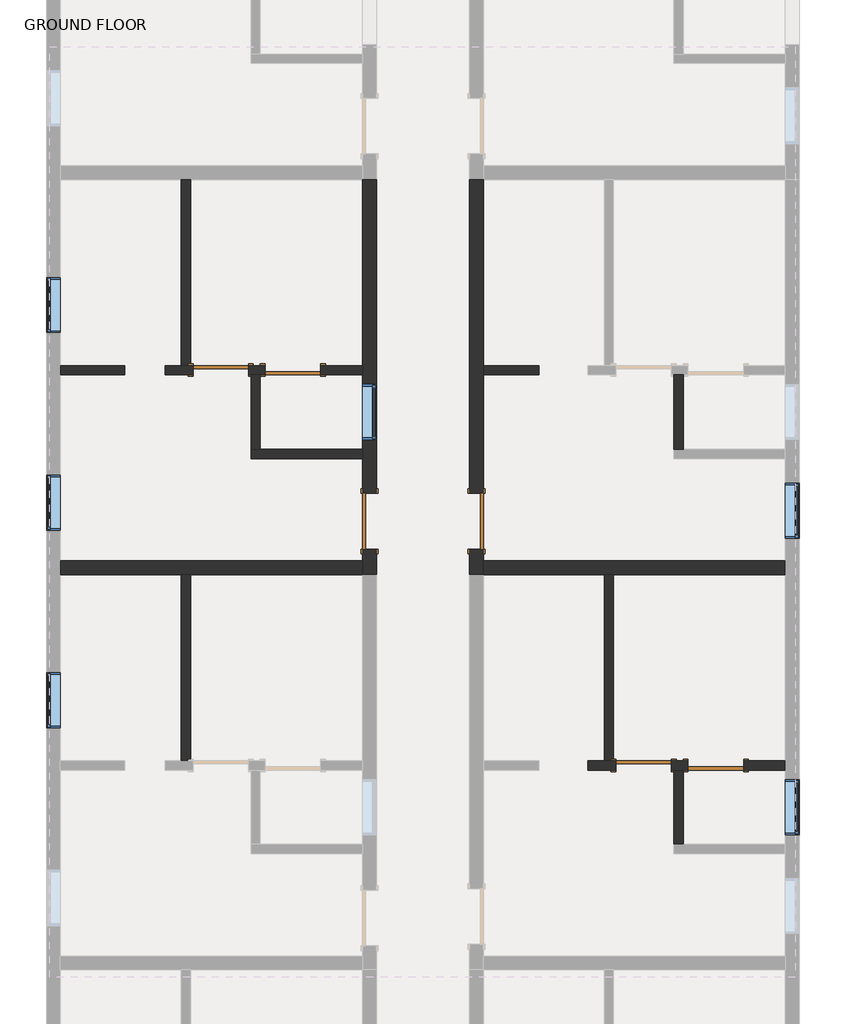
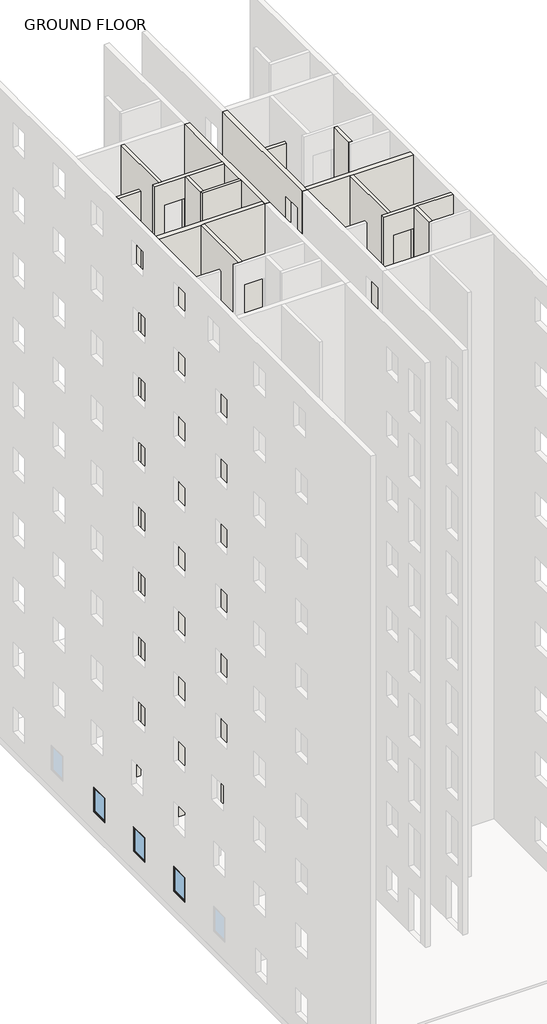
# One storey, part 5 of 7: 15 walls, 6 doors, 6 windows.
"""IFC4 building model written with IfcOpenShell, lengths in millimetres."""

from ifc_helpers import new_model, si_unit, origin, origin_with_axes, place, context, project, spatial, polyline, outline, extrude, faceted_brep, transform, mapped, element, save
from components import door_686f89d2, door_16372e1c, door_a90ba1ad, door_0ca8825f, window_c1f32544

model = new_model("IFC4")

# Units and contexts
model_context = context("Model", 3, world=origin())
ifc_project = project(units=[si_unit("LENGTHUNIT", "METRE", prefix="MILLI")], contexts=[model_context])

# Site, building, storey
site = spatial("IfcSite", under=ifc_project)
building = spatial("IfcBuilding", under=site)
storey = spatial("IfcBuildingStorey", under=building, Name="GROUND FLOOR", Elevation=0.0)

# Doors
placement = place(None, origin())
door_shape = door_686f89d2(model_context)
element("IfcDoor", 1, ObjectType="Single-Flush : 36\" x 84\"", at=placement, inside=storey, context=model_context, shape_type="MappedRepresentation", body=[
    mapped(door_shape, transform((-9863.5902461, 5475.2710592, 0.0), x_axis=(-1.0, 0.0, 0.0), y_axis=(0.0, -1.0, 0.0), z_axis=(0.0, 0.0, 1.0))),
])
element("IfcDoor", 2, ObjectType="Single-Flush : 36\" x 84\"", at=placement, inside=storey, context=model_context, shape_type="MappedRepresentation", body=[
    mapped(door_shape, transform((-2929.3902461, -1001.7289408, 0.0), x_axis=(-1.0, 0.0, 0.0), y_axis=(0.0, -1.0, 0.0), z_axis=(0.0, 0.0, 1.0))),
])
door_2_shape = door_16372e1c(model_context)
element("IfcDoor", 3, ObjectType="Single-Flush : 36\" x 84\"", at=placement, inside=storey, context=model_context, shape_type="MappedRepresentation", body=[
    mapped(door_2_shape, transform((-8682.4902461, 5475.2710592, 0.0), x_axis=(-1.0, 0.0, 0.0), y_axis=(0.0, -1.0, 0.0), z_axis=(0.0, 0.0, 1.0))),
])
element("IfcDoor", 4, ObjectType="Single-Flush : 36\" x 84\"", at=placement, inside=storey, context=model_context, shape_type="MappedRepresentation", body=[
    mapped(door_2_shape, transform((-1748.2902461, -1001.7289408, 0.0), x_axis=(-1.0, 0.0, 0.0), y_axis=(0.0, -1.0, 0.0), z_axis=(0.0, 0.0, 1.0))),
])
door_3_shape = door_a90ba1ad(model_context)
element("IfcDoor", 5, ObjectType="Single-Flush : 36\" x 84\"", at=placement, inside=storey, context=model_context, shape_type="MappedRepresentation", body=[
    mapped(door_3_shape, transform((-7425.1902461, 2998.7710592, 0.0), x_axis=(0.0, -1.0, 0.0), y_axis=(1.0, 0.0, 0.0), z_axis=(0.0, 0.0, 1.0))),
])
door_4_shape = door_0ca8825f(model_context)
element("IfcDoor", 6, ObjectType="Single-Flush : 36\" x 84\"", at=placement, inside=storey, context=model_context, shape_type="MappedRepresentation", body=[
    mapped(door_4_shape, transform((-5672.5902461, 2998.7710592, 0.0), x_axis=(0.0, -1.0, 0.0), y_axis=(1.0, 0.0, 0.0), z_axis=(0.0, 0.0, 1.0))),
])

# Walls
element("IfcWall", 7, ObjectType="Generic - 8\"", at=placement, inside=storey, context=model_context, shape_type="Brep", body=[
    faceted_brep([(-5558.2902461, 2122.4710592, 0.0), (-5558.2902461, 2351.0710592, 0.0), (-5558.2902461, 2541.5710592, 0.0), (-5558.2902461, 2541.5710592, 2133.6), (-5558.2902461, 3455.9710592, 2133.6), (-5558.2902461, 3455.9710592, 0.0), (-5558.2902461, 5399.0710592, 0.0), (-5558.2902461, 5551.4710592, 0.0), (-5558.2902461, 8599.4710592, 0.0), (-5558.2902461, 8599.4710592, 32004.0), (-5558.2902461, 5551.4710592, 32004.0), (-5558.2902461, 5399.0710592, 32004.0), (-5558.2902461, 2351.0710592, 32004.0), (-5558.2902461, 2122.4710592, 32004.0), (-5558.2902461, 3455.9710592, 3200.4), (-5558.2902461, 2541.5710592, 3200.4), (-5558.2902461, 2541.5710592, 5334.0), (-5558.2902461, 3455.9710592, 5334.0), (-5558.2902461, 3455.9710592, 6400.8), (-5558.2902461, 2541.5710592, 6400.8), (-5558.2902461, 2541.5710592, 8534.4), (-5558.2902461, 3455.9710592, 8534.4), (-5558.2902461, 3455.9710592, 9601.2), (-5558.2902461, 2541.5710592, 9601.2), (-5558.2902461, 2541.5710592, 11734.8), (-5558.2902461, 3455.9710592, 11734.8), (-5558.2902461, 3455.9710592, 12801.6), (-5558.2902461, 2541.5710592, 12801.6), (-5558.2902461, 2541.5710592, 14935.2), (-5558.2902461, 3455.9710592, 14935.2), (-5558.2902461, 3455.9710592, 19202.4), (-5558.2902461, 2541.5710592, 19202.4), (-5558.2902461, 2541.5710592, 21336.0), (-5558.2902461, 3455.9710592, 21336.0), (-5558.2902461, 3455.9710592, 22402.8), (-5558.2902461, 2541.5710592, 22402.8), (-5558.2902461, 2541.5710592, 24536.4), (-5558.2902461, 3455.9710592, 24536.4), (-5558.2902461, 3455.9710592, 25603.2), (-5558.2902461, 2541.5710592, 25603.2), (-5558.2902461, 2541.5710592, 27736.8), (-5558.2902461, 3455.9710592, 27736.8), (-5558.2902461, 3455.9710592, 28803.6), (-5558.2902461, 2541.5710592, 28803.6), (-5558.2902461, 2541.5710592, 30937.2), (-5558.2902461, 3455.9710592, 30937.2), (-5786.8902461, 2541.5710592, 2133.6), (-5786.8902461, 2541.5710592, 0.0), (-5786.8902461, 2122.4710592, 0.0), (-5786.8902461, 2122.4710592, 32004.0), (-5786.8902461, 8599.4710592, 32004.0), (-5786.8902461, 8599.4710592, 0.0), (-5786.8902461, 3455.9710592, 0.0), (-5786.8902461, 3455.9710592, 2133.6), (-5786.8902461, 3455.9710592, 3200.4), (-5786.8902461, 3455.9710592, 5334.0), (-5786.8902461, 2541.5710592, 5334.0), (-5786.8902461, 2541.5710592, 3200.4), (-5786.8902461, 3455.9710592, 6400.8), (-5786.8902461, 3455.9710592, 8534.4), (-5786.8902461, 2541.5710592, 8534.4), (-5786.8902461, 2541.5710592, 6400.8), (-5786.8902461, 3455.9710592, 9601.2), (-5786.8902461, 3455.9710592, 11734.8), (-5786.8902461, 2541.5710592, 11734.8), (-5786.8902461, 2541.5710592, 9601.2), (-5786.8902461, 3455.9710592, 12801.6), (-5786.8902461, 3455.9710592, 14935.2), (-5786.8902461, 2541.5710592, 14935.2), (-5786.8902461, 2541.5710592, 12801.6), (-5786.8902461, 3455.9710592, 19202.4), (-5786.8902461, 3455.9710592, 21336.0), (-5786.8902461, 2541.5710592, 21336.0), (-5786.8902461, 2541.5710592, 19202.4), (-5786.8902461, 3455.9710592, 22402.8), (-5786.8902461, 3455.9710592, 24536.4), (-5786.8902461, 2541.5710592, 24536.4), (-5786.8902461, 2541.5710592, 22402.8), (-5786.8902461, 3455.9710592, 25603.2), (-5786.8902461, 3455.9710592, 27736.8), (-5786.8902461, 2541.5710592, 27736.8), (-5786.8902461, 2541.5710592, 25603.2), (-5786.8902461, 3455.9710592, 28803.6), (-5786.8902461, 3455.9710592, 30937.2), (-5786.8902461, 2541.5710592, 30937.2), (-5786.8902461, 2541.5710592, 28803.6)], [[[0, 1, 2, 3, 4, 5, 6, 7, 8, 9, 10, 11, 12, 13], [14, 15, 16, 17], [18, 19, 20, 21], [22, 23, 24, 25], [26, 27, 28, 29], [30, 31, 32, 33], [34, 35, 36, 37], [38, 39, 40, 41], [42, 43, 44, 45]], [[46, 47, 48, 49, 50, 51, 52, 53], [54, 55, 56, 57], [58, 59, 60, 61], [62, 63, 64, 65], [66, 67, 68, 69], [70, 71, 72, 73], [74, 75, 76, 77], [78, 79, 80, 81], [82, 83, 84, 85]], [[52, 51, 8, 7, 6, 5]], [[48, 47, 2, 1, 0]], [[13, 12, 11, 10, 9, 50, 49]], [[0, 13, 49, 48]], [[9, 8, 51, 50]], [[3, 2, 47, 46]], [[4, 3, 46, 53]], [[5, 4, 53, 52]], [[15, 14, 54, 57]], [[16, 15, 57, 56]], [[17, 16, 56, 55]], [[14, 17, 55, 54]], [[19, 18, 58, 61]], [[20, 19, 61, 60]], [[21, 20, 60, 59]], [[18, 21, 59, 58]], [[23, 22, 62, 65]], [[24, 23, 65, 64]], [[25, 24, 64, 63]], [[22, 25, 63, 62]], [[27, 26, 66, 69]], [[28, 27, 69, 68]], [[29, 28, 68, 67]], [[26, 29, 67, 66]], [[31, 30, 70, 73]], [[32, 31, 73, 72]], [[33, 32, 72, 71]], [[30, 33, 71, 70]], [[35, 34, 74, 77]], [[36, 35, 77, 76]], [[37, 36, 76, 75]], [[34, 37, 75, 74]], [[39, 38, 78, 81]], [[40, 39, 81, 80]], [[41, 40, 80, 79]], [[38, 41, 79, 78]], [[43, 42, 82, 85]], [[44, 43, 85, 84]], [[45, 44, 84, 83]], [[42, 45, 83, 82]]]),
])
element("IfcWall", 8, ObjectType="INNER WALL 2", at=placement, inside=storey, context=model_context, shape_type="SweptSolid", body=[
    extrude(outline(polyline([(-2281.6902461, 5399.0710592), (-2281.6902461, 4179.8710592), (-2434.0902461, 4179.8710592), (-2434.0902461, 5399.0710592), (-2281.6902461, 5399.0710592)])), origin_with_axes(), (0.0, 0.0, 1.0), 32004.0),
])
element("IfcWall", 9, ObjectType="INNER WALL 2", at=placement, inside=storey, context=model_context, shape_type="Brep", body=[
    faceted_brep([(-2472.1902461, -1077.9289408, 0.0), (-2434.0902461, -1077.9289408, 0.0), (-2281.6902461, -1077.9289408, 0.0), (-2205.4902461, -1077.9289408, 0.0), (-2205.4902461, -1077.9289408, 2133.6), (-1291.0902461, -1077.9289408, 2133.6), (-1291.0902461, -1077.9289408, 0.0), (-605.2902461, -1077.9289408, 0.0), (-605.2902461, -1077.9289408, 32004.0), (-2281.6902461, -1077.9289408, 32004.0), (-2434.0902461, -1077.9289408, 32004.0), (-3843.7902461, -1077.9289408, 32004.0), (-3843.7902461, -1077.9289408, 0.0), (-3386.5902461, -1077.9289408, 0.0), (-3386.5902461, -1077.9289408, 2133.6), (-2472.1902461, -1077.9289408, 2133.6), (-1291.0902461, -1077.9289408, 3200.4), (-2205.4902461, -1077.9289408, 3200.4), (-2205.4902461, -1077.9289408, 5334.0), (-1291.0902461, -1077.9289408, 5334.0), (-2472.1902461, -1077.9289408, 3200.4), (-3386.5902461, -1077.9289408, 3200.4), (-3386.5902461, -1077.9289408, 5334.0), (-2472.1902461, -1077.9289408, 5334.0), (-2472.1902461, -1077.9289408, 6400.8), (-3386.5902461, -1077.9289408, 6400.8), (-3386.5902461, -1077.9289408, 8534.4), (-2472.1902461, -1077.9289408, 8534.4), (-1291.0902461, -1077.9289408, 6400.8), (-2205.4902461, -1077.9289408, 6400.8), (-2205.4902461, -1077.9289408, 8534.4), (-1291.0902461, -1077.9289408, 8534.4), (-2472.1902461, -1077.9289408, 9601.2), (-3386.5902461, -1077.9289408, 9601.2), (-3386.5902461, -1077.9289408, 11734.8), (-2472.1902461, -1077.9289408, 11734.8), (-1291.0902461, -1077.9289408, 9601.2), (-2205.4902461, -1077.9289408, 9601.2), (-2205.4902461, -1077.9289408, 11734.8), (-1291.0902461, -1077.9289408, 11734.8), (-1291.0902461, -1077.9289408, 12801.6), (-2205.4902461, -1077.9289408, 12801.6), (-2205.4902461, -1077.9289408, 14935.2), (-1291.0902461, -1077.9289408, 14935.2), (-2472.1902461, -1077.9289408, 12801.6), (-3386.5902461, -1077.9289408, 12801.6), (-3386.5902461, -1077.9289408, 14935.2), (-2472.1902461, -1077.9289408, 14935.2), (-2472.1902461, -1077.9289408, 16002.0), (-3386.5902461, -1077.9289408, 16002.0), (-3386.5902461, -1077.9289408, 18135.6), (-2472.1902461, -1077.9289408, 18135.6), (-1291.0902461, -1077.9289408, 16002.0), (-2205.4902461, -1077.9289408, 16002.0), (-2205.4902461, -1077.9289408, 18135.6), (-1291.0902461, -1077.9289408, 18135.6), (-1291.0902461, -1077.9289408, 19202.4), (-2205.4902461, -1077.9289408, 19202.4), (-2205.4902461, -1077.9289408, 21336.0), (-1291.0902461, -1077.9289408, 21336.0), (-2472.1902461, -1077.9289408, 19202.4), (-3386.5902461, -1077.9289408, 19202.4), (-3386.5902461, -1077.9289408, 21336.0), (-2472.1902461, -1077.9289408, 21336.0), (-1291.0902461, -1077.9289408, 22402.8), (-2205.4902461, -1077.9289408, 22402.8), (-2205.4902461, -1077.9289408, 24536.4), (-1291.0902461, -1077.9289408, 24536.4), (-2472.1902461, -1077.9289408, 22402.8), (-3386.5902461, -1077.9289408, 22402.8), (-3386.5902461, -1077.9289408, 24536.4), (-2472.1902461, -1077.9289408, 24536.4), (-2472.1902461, -1077.9289408, 25603.2), (-3386.5902461, -1077.9289408, 25603.2), (-3386.5902461, -1077.9289408, 27736.8), (-2472.1902461, -1077.9289408, 27736.8), (-1291.0902461, -1077.9289408, 25603.2), (-2205.4902461, -1077.9289408, 25603.2), (-2205.4902461, -1077.9289408, 27736.8), (-1291.0902461, -1077.9289408, 27736.8), (-2472.1902461, -1077.9289408, 28803.6), (-3386.5902461, -1077.9289408, 28803.6), (-3386.5902461, -1077.9289408, 30937.2), (-2472.1902461, -1077.9289408, 30937.2), (-1291.0902461, -1077.9289408, 28803.6), (-2205.4902461, -1077.9289408, 28803.6), (-2205.4902461, -1077.9289408, 30937.2), (-1291.0902461, -1077.9289408, 30937.2), (-2205.4902461, -925.5289408, 2133.6), (-2205.4902461, -925.5289408, 0.0), (-2472.1902461, -925.5289408, 0.0), (-2472.1902461, -925.5289408, 2133.6), (-3386.5902461, -925.5289408, 2133.6), (-3386.5902461, -925.5289408, 0.0), (-3424.6902461, -925.5289408, 0.0), (-3577.0902461, -925.5289408, 0.0), (-3843.7902461, -925.5289408, 0.0), (-3843.7902461, -925.5289408, 32004.0), (-3577.0902461, -925.5289408, 32004.0), (-3424.6902461, -925.5289408, 32004.0), (-605.2902461, -925.5289408, 32004.0), (-605.2902461, -925.5289408, 0.0), (-1291.0902461, -925.5289408, 0.0), (-1291.0902461, -925.5289408, 2133.6), (-1291.0902461, -925.5289408, 3200.4), (-1291.0902461, -925.5289408, 5334.0), (-2205.4902461, -925.5289408, 5334.0), (-2205.4902461, -925.5289408, 3200.4), (-2472.1902461, -925.5289408, 3200.4), (-2472.1902461, -925.5289408, 5334.0), (-3386.5902461, -925.5289408, 5334.0), (-3386.5902461, -925.5289408, 3200.4), (-2472.1902461, -925.5289408, 6400.8), (-2472.1902461, -925.5289408, 8534.4), (-3386.5902461, -925.5289408, 8534.4), (-3386.5902461, -925.5289408, 6400.8), (-1291.0902461, -925.5289408, 6400.8), (-1291.0902461, -925.5289408, 8534.4), (-2205.4902461, -925.5289408, 8534.4), (-2205.4902461, -925.5289408, 6400.8), (-2472.1902461, -925.5289408, 9601.2), (-2472.1902461, -925.5289408, 11734.8), (-3386.5902461, -925.5289408, 11734.8), (-3386.5902461, -925.5289408, 9601.2), (-1291.0902461, -925.5289408, 9601.2), (-1291.0902461, -925.5289408, 11734.8), (-2205.4902461, -925.5289408, 11734.8), (-2205.4902461, -925.5289408, 9601.2), (-1291.0902461, -925.5289408, 12801.6), (-1291.0902461, -925.5289408, 14935.2), (-2205.4902461, -925.5289408, 14935.2), (-2205.4902461, -925.5289408, 12801.6), (-2472.1902461, -925.5289408, 12801.6), (-2472.1902461, -925.5289408, 14935.2), (-3386.5902461, -925.5289408, 14935.2), (-3386.5902461, -925.5289408, 12801.6), (-2472.1902461, -925.5289408, 16002.0), (-2472.1902461, -925.5289408, 18135.6), (-3386.5902461, -925.5289408, 18135.6), (-3386.5902461, -925.5289408, 16002.0), (-1291.0902461, -925.5289408, 16002.0), (-1291.0902461, -925.5289408, 18135.6), (-2205.4902461, -925.5289408, 18135.6), (-2205.4902461, -925.5289408, 16002.0), (-1291.0902461, -925.5289408, 19202.4), (-1291.0902461, -925.5289408, 21336.0), (-2205.4902461, -925.5289408, 21336.0), (-2205.4902461, -925.5289408, 19202.4), (-2472.1902461, -925.5289408, 19202.4), (-2472.1902461, -925.5289408, 21336.0), (-3386.5902461, -925.5289408, 21336.0), (-3386.5902461, -925.5289408, 19202.4), (-1291.0902461, -925.5289408, 22402.8), (-1291.0902461, -925.5289408, 24536.4), (-2205.4902461, -925.5289408, 24536.4), (-2205.4902461, -925.5289408, 22402.8), (-2472.1902461, -925.5289408, 22402.8), (-2472.1902461, -925.5289408, 24536.4), (-3386.5902461, -925.5289408, 24536.4), (-3386.5902461, -925.5289408, 22402.8), (-2472.1902461, -925.5289408, 25603.2), (-2472.1902461, -925.5289408, 27736.8), (-3386.5902461, -925.5289408, 27736.8), (-3386.5902461, -925.5289408, 25603.2), (-1291.0902461, -925.5289408, 25603.2), (-1291.0902461, -925.5289408, 27736.8), (-2205.4902461, -925.5289408, 27736.8), (-2205.4902461, -925.5289408, 25603.2), (-2472.1902461, -925.5289408, 28803.6), (-2472.1902461, -925.5289408, 30937.2), (-3386.5902461, -925.5289408, 30937.2), (-3386.5902461, -925.5289408, 28803.6), (-1291.0902461, -925.5289408, 28803.6), (-1291.0902461, -925.5289408, 30937.2), (-2205.4902461, -925.5289408, 30937.2), (-2205.4902461, -925.5289408, 28803.6)], [[[0, 1, 2, 3, 4, 5, 6, 7, 8, 9, 10, 11, 12, 13, 14, 15], [16, 17, 18, 19], [20, 21, 22, 23], [24, 25, 26, 27], [28, 29, 30, 31], [32, 33, 34, 35], [36, 37, 38, 39], [40, 41, 42, 43], [44, 45, 46, 47], [48, 49, 50, 51], [52, 53, 54, 55], [56, 57, 58, 59], [60, 61, 62, 63], [64, 65, 66, 67], [68, 69, 70, 71], [72, 73, 74, 75], [76, 77, 78, 79], [80, 81, 82, 83], [84, 85, 86, 87]], [[88, 89, 90, 91, 92, 93, 94, 95, 96, 97, 98, 99, 100, 101, 102, 103], [104, 105, 106, 107], [108, 109, 110, 111], [112, 113, 114, 115], [116, 117, 118, 119], [120, 121, 122, 123], [124, 125, 126, 127], [128, 129, 130, 131], [132, 133, 134, 135], [136, 137, 138, 139], [140, 141, 142, 143], [144, 145, 146, 147], [148, 149, 150, 151], [152, 153, 154, 155], [156, 157, 158, 159], [160, 161, 162, 163], [164, 165, 166, 167], [168, 169, 170, 171], [172, 173, 174, 175]], [[96, 95, 94, 93, 13, 12]], [[102, 101, 7, 6]], [[90, 89, 3, 2, 1, 0]], [[11, 10, 9, 8, 100, 99, 98, 97]], [[12, 11, 97, 96]], [[8, 7, 101, 100]], [[14, 13, 93, 92]], [[15, 14, 92, 91]], [[0, 15, 91, 90]], [[4, 3, 89, 88]], [[5, 4, 88, 103]], [[6, 5, 103, 102]], [[17, 16, 104, 107]], [[18, 17, 107, 106]], [[19, 18, 106, 105]], [[16, 19, 105, 104]], [[21, 20, 108, 111]], [[22, 21, 111, 110]], [[23, 22, 110, 109]], [[20, 23, 109, 108]], [[25, 24, 112, 115]], [[26, 25, 115, 114]], [[27, 26, 114, 113]], [[24, 27, 113, 112]], [[29, 28, 116, 119]], [[30, 29, 119, 118]], [[31, 30, 118, 117]], [[28, 31, 117, 116]], [[33, 32, 120, 123]], [[34, 33, 123, 122]], [[35, 34, 122, 121]], [[32, 35, 121, 120]], [[37, 36, 124, 127]], [[38, 37, 127, 126]], [[39, 38, 126, 125]], [[36, 39, 125, 124]], [[41, 40, 128, 131]], [[42, 41, 131, 130]], [[43, 42, 130, 129]], [[40, 43, 129, 128]], [[45, 44, 132, 135]], [[46, 45, 135, 134]], [[47, 46, 134, 133]], [[44, 47, 133, 132]], [[49, 48, 136, 139]], [[50, 49, 139, 138]], [[51, 50, 138, 137]], [[48, 51, 137, 136]], [[53, 52, 140, 143]], [[54, 53, 143, 142]], [[55, 54, 142, 141]], [[52, 55, 141, 140]], [[57, 56, 144, 147]], [[58, 57, 147, 146]], [[59, 58, 146, 145]], [[56, 59, 145, 144]], [[61, 60, 148, 151]], [[62, 61, 151, 150]], [[63, 62, 150, 149]], [[60, 63, 149, 148]], [[65, 64, 152, 155]], [[66, 65, 155, 154]], [[67, 66, 154, 153]], [[64, 67, 153, 152]], [[69, 68, 156, 159]], [[70, 69, 159, 158]], [[71, 70, 158, 157]], [[68, 71, 157, 156]], [[73, 72, 160, 163]], [[74, 73, 163, 162]], [[75, 74, 162, 161]], [[72, 75, 161, 160]], [[77, 76, 164, 167]], [[78, 77, 167, 166]], [[79, 78, 166, 165]], [[76, 79, 165, 164]], [[81, 80, 168, 171]], [[82, 81, 171, 170]], [[83, 82, 170, 169]], [[80, 83, 169, 168]], [[85, 84, 172, 175]], [[86, 85, 175, 174]], [[87, 86, 174, 173]], [[84, 87, 173, 172]]]),
])
element("IfcWall", 10, ObjectType="INNER WALL 2", at=placement, inside=storey, context=model_context, shape_type="SweptSolid", body=[
    extrude(outline(polyline([(-3424.6902461, 2122.4710592), (-3424.6902461, -925.5289408), (-3577.0902461, -925.5289408), (-3577.0902461, 2122.4710592), (-3424.6902461, 2122.4710592)])), origin_with_axes(), (0.0, 0.0, 1.0), 32004.0),
])
element("IfcWall", 11, ObjectType="INNER WALL 2", at=placement, inside=storey, context=model_context, shape_type="SweptSolid", body=[
    extrude(outline(polyline([(-2281.6902461, -1077.9289408), (-2281.6902461, -2297.1289408), (-2434.0902461, -2297.1289408), (-2434.0902461, -1077.9289408), (-2281.6902461, -1077.9289408)])), origin_with_axes(), (0.0, 0.0, 1.0), 32004.0),
])
element("IfcWall", 12, ObjectType="INNER WALL 2", at=placement, inside=storey, context=model_context, shape_type="Brep", body=[
    faceted_brep([(-9406.3902461, 5399.0710592, 0.0), (-9368.2902461, 5399.0710592, 0.0), (-9215.8902461, 5399.0710592, 0.0), (-9139.6902461, 5399.0710592, 0.0), (-9139.6902461, 5399.0710592, 2133.6), (-8225.2902461, 5399.0710592, 2133.6), (-8225.2902461, 5399.0710592, 0.0), (-7539.4902461, 5399.0710592, 0.0), (-7539.4902461, 5399.0710592, 32004.0), (-9215.8902461, 5399.0710592, 32004.0), (-9368.2902461, 5399.0710592, 32004.0), (-10777.9902461, 5399.0710592, 32004.0), (-10777.9902461, 5399.0710592, 0.0), (-10320.7902461, 5399.0710592, 0.0), (-10320.7902461, 5399.0710592, 2133.6), (-9406.3902461, 5399.0710592, 2133.6), (-9406.3902461, 5399.0710592, 3200.4), (-10320.7902461, 5399.0710592, 3200.4), (-10320.7902461, 5399.0710592, 5334.0), (-9406.3902461, 5399.0710592, 5334.0), (-8225.2902461, 5399.0710592, 3200.4), (-9139.6902461, 5399.0710592, 3200.4), (-9139.6902461, 5399.0710592, 5334.0), (-8225.2902461, 5399.0710592, 5334.0), (-9406.3902461, 5399.0710592, 6400.8), (-10320.7902461, 5399.0710592, 6400.8), (-10320.7902461, 5399.0710592, 8534.4), (-9406.3902461, 5399.0710592, 8534.4), (-8225.2902461, 5399.0710592, 6400.8), (-9139.6902461, 5399.0710592, 6400.8), (-9139.6902461, 5399.0710592, 8534.4), (-8225.2902461, 5399.0710592, 8534.4), (-9406.3902461, 5399.0710592, 9601.2), (-10320.7902461, 5399.0710592, 9601.2), (-10320.7902461, 5399.0710592, 11734.8), (-9406.3902461, 5399.0710592, 11734.8), (-8225.2902461, 5399.0710592, 9601.2), (-9139.6902461, 5399.0710592, 9601.2), (-9139.6902461, 5399.0710592, 11734.8), (-8225.2902461, 5399.0710592, 11734.8), (-9406.3902461, 5399.0710592, 12801.6), (-10320.7902461, 5399.0710592, 12801.6), (-10320.7902461, 5399.0710592, 14935.2), (-9406.3902461, 5399.0710592, 14935.2), (-8225.2902461, 5399.0710592, 12801.6), (-9139.6902461, 5399.0710592, 12801.6), (-9139.6902461, 5399.0710592, 14935.2), (-8225.2902461, 5399.0710592, 14935.2), (-9406.3902461, 5399.0710592, 16002.0), (-10320.7902461, 5399.0710592, 16002.0), (-10320.7902461, 5399.0710592, 18135.6), (-9406.3902461, 5399.0710592, 18135.6), (-8225.2902461, 5399.0710592, 16002.0), (-9139.6902461, 5399.0710592, 16002.0), (-9139.6902461, 5399.0710592, 18135.6), (-8225.2902461, 5399.0710592, 18135.6), (-9406.3902461, 5399.0710592, 19202.4), (-10320.7902461, 5399.0710592, 19202.4), (-10320.7902461, 5399.0710592, 21336.0), (-9406.3902461, 5399.0710592, 21336.0), (-8225.2902461, 5399.0710592, 19202.4), (-9139.6902461, 5399.0710592, 19202.4), (-9139.6902461, 5399.0710592, 21336.0), (-8225.2902461, 5399.0710592, 21336.0), (-9406.3902461, 5399.0710592, 22402.8), (-10320.7902461, 5399.0710592, 22402.8), (-10320.7902461, 5399.0710592, 24536.4), (-9406.3902461, 5399.0710592, 24536.4), (-8225.2902461, 5399.0710592, 22402.8), (-9139.6902461, 5399.0710592, 22402.8), (-9139.6902461, 5399.0710592, 24536.4), (-8225.2902461, 5399.0710592, 24536.4), (-9406.3902461, 5399.0710592, 25603.2), (-10320.7902461, 5399.0710592, 25603.2), (-10320.7902461, 5399.0710592, 27736.8), (-9406.3902461, 5399.0710592, 27736.8), (-8225.2902461, 5399.0710592, 25603.2), (-9139.6902461, 5399.0710592, 25603.2), (-9139.6902461, 5399.0710592, 27736.8), (-8225.2902461, 5399.0710592, 27736.8), (-9406.3902461, 5399.0710592, 28803.6), (-10320.7902461, 5399.0710592, 28803.6), (-10320.7902461, 5399.0710592, 30937.2), (-9406.3902461, 5399.0710592, 30937.2), (-8225.2902461, 5399.0710592, 28803.6), (-9139.6902461, 5399.0710592, 28803.6), (-9139.6902461, 5399.0710592, 30937.2), (-8225.2902461, 5399.0710592, 30937.2), (-9139.6902461, 5551.4710592, 2133.6), (-9139.6902461, 5551.4710592, 0.0), (-9406.3902461, 5551.4710592, 0.0), (-9406.3902461, 5551.4710592, 2133.6), (-10320.7902461, 5551.4710592, 2133.6), (-10320.7902461, 5551.4710592, 0.0), (-10358.8902461, 5551.4710592, 0.0), (-10511.2902461, 5551.4710592, 0.0), (-10777.9902461, 5551.4710592, 0.0), (-10777.9902461, 5551.4710592, 32004.0), (-10511.2902461, 5551.4710592, 32004.0), (-10358.8902461, 5551.4710592, 32004.0), (-7539.4902461, 5551.4710592, 32004.0), (-7539.4902461, 5551.4710592, 0.0), (-8225.2902461, 5551.4710592, 0.0), (-8225.2902461, 5551.4710592, 2133.6), (-9406.3902461, 5551.4710592, 3200.4), (-9406.3902461, 5551.4710592, 5334.0), (-10320.7902461, 5551.4710592, 5334.0), (-10320.7902461, 5551.4710592, 3200.4), (-8225.2902461, 5551.4710592, 3200.4), (-8225.2902461, 5551.4710592, 5334.0), (-9139.6902461, 5551.4710592, 5334.0), (-9139.6902461, 5551.4710592, 3200.4), (-9406.3902461, 5551.4710592, 6400.8), (-9406.3902461, 5551.4710592, 8534.4), (-10320.7902461, 5551.4710592, 8534.4), (-10320.7902461, 5551.4710592, 6400.8), (-8225.2902461, 5551.4710592, 6400.8), (-8225.2902461, 5551.4710592, 8534.4), (-9139.6902461, 5551.4710592, 8534.4), (-9139.6902461, 5551.4710592, 6400.8), (-9406.3902461, 5551.4710592, 9601.2), (-9406.3902461, 5551.4710592, 11734.8), (-10320.7902461, 5551.4710592, 11734.8), (-10320.7902461, 5551.4710592, 9601.2), (-8225.2902461, 5551.4710592, 9601.2), (-8225.2902461, 5551.4710592, 11734.8), (-9139.6902461, 5551.4710592, 11734.8), (-9139.6902461, 5551.4710592, 9601.2), (-9406.3902461, 5551.4710592, 12801.6), (-9406.3902461, 5551.4710592, 14935.2), (-10320.7902461, 5551.4710592, 14935.2), (-10320.7902461, 5551.4710592, 12801.6), (-8225.2902461, 5551.4710592, 12801.6), (-8225.2902461, 5551.4710592, 14935.2), (-9139.6902461, 5551.4710592, 14935.2), (-9139.6902461, 5551.4710592, 12801.6), (-9406.3902461, 5551.4710592, 16002.0), (-9406.3902461, 5551.4710592, 18135.6), (-10320.7902461, 5551.4710592, 18135.6), (-10320.7902461, 5551.4710592, 16002.0), (-8225.2902461, 5551.4710592, 16002.0), (-8225.2902461, 5551.4710592, 18135.6), (-9139.6902461, 5551.4710592, 18135.6), (-9139.6902461, 5551.4710592, 16002.0), (-9406.3902461, 5551.4710592, 19202.4), (-9406.3902461, 5551.4710592, 21336.0), (-10320.7902461, 5551.4710592, 21336.0), (-10320.7902461, 5551.4710592, 19202.4), (-8225.2902461, 5551.4710592, 19202.4), (-8225.2902461, 5551.4710592, 21336.0), (-9139.6902461, 5551.4710592, 21336.0), (-9139.6902461, 5551.4710592, 19202.4), (-9406.3902461, 5551.4710592, 22402.8), (-9406.3902461, 5551.4710592, 24536.4), (-10320.7902461, 5551.4710592, 24536.4), (-10320.7902461, 5551.4710592, 22402.8), (-8225.2902461, 5551.4710592, 22402.8), (-8225.2902461, 5551.4710592, 24536.4), (-9139.6902461, 5551.4710592, 24536.4), (-9139.6902461, 5551.4710592, 22402.8), (-9406.3902461, 5551.4710592, 25603.2), (-9406.3902461, 5551.4710592, 27736.8), (-10320.7902461, 5551.4710592, 27736.8), (-10320.7902461, 5551.4710592, 25603.2), (-8225.2902461, 5551.4710592, 25603.2), (-8225.2902461, 5551.4710592, 27736.8), (-9139.6902461, 5551.4710592, 27736.8), (-9139.6902461, 5551.4710592, 25603.2), (-9406.3902461, 5551.4710592, 28803.6), (-9406.3902461, 5551.4710592, 30937.2), (-10320.7902461, 5551.4710592, 30937.2), (-10320.7902461, 5551.4710592, 28803.6), (-8225.2902461, 5551.4710592, 28803.6), (-8225.2902461, 5551.4710592, 30937.2), (-9139.6902461, 5551.4710592, 30937.2), (-9139.6902461, 5551.4710592, 28803.6)], [[[0, 1, 2, 3, 4, 5, 6, 7, 8, 9, 10, 11, 12, 13, 14, 15], [16, 17, 18, 19], [20, 21, 22, 23], [24, 25, 26, 27], [28, 29, 30, 31], [32, 33, 34, 35], [36, 37, 38, 39], [40, 41, 42, 43], [44, 45, 46, 47], [48, 49, 50, 51], [52, 53, 54, 55], [56, 57, 58, 59], [60, 61, 62, 63], [64, 65, 66, 67], [68, 69, 70, 71], [72, 73, 74, 75], [76, 77, 78, 79], [80, 81, 82, 83], [84, 85, 86, 87]], [[88, 89, 90, 91, 92, 93, 94, 95, 96, 97, 98, 99, 100, 101, 102, 103], [104, 105, 106, 107], [108, 109, 110, 111], [112, 113, 114, 115], [116, 117, 118, 119], [120, 121, 122, 123], [124, 125, 126, 127], [128, 129, 130, 131], [132, 133, 134, 135], [136, 137, 138, 139], [140, 141, 142, 143], [144, 145, 146, 147], [148, 149, 150, 151], [152, 153, 154, 155], [156, 157, 158, 159], [160, 161, 162, 163], [164, 165, 166, 167], [168, 169, 170, 171], [172, 173, 174, 175]], [[96, 95, 94, 93, 13, 12]], [[102, 101, 7, 6]], [[90, 89, 3, 2, 1, 0]], [[11, 10, 9, 8, 100, 99, 98, 97]], [[12, 11, 97, 96]], [[8, 7, 101, 100]], [[14, 13, 93, 92]], [[15, 14, 92, 91]], [[0, 15, 91, 90]], [[4, 3, 89, 88]], [[5, 4, 88, 103]], [[6, 5, 103, 102]], [[17, 16, 104, 107]], [[18, 17, 107, 106]], [[19, 18, 106, 105]], [[16, 19, 105, 104]], [[21, 20, 108, 111]], [[22, 21, 111, 110]], [[23, 22, 110, 109]], [[20, 23, 109, 108]], [[25, 24, 112, 115]], [[26, 25, 115, 114]], [[27, 26, 114, 113]], [[24, 27, 113, 112]], [[29, 28, 116, 119]], [[30, 29, 119, 118]], [[31, 30, 118, 117]], [[28, 31, 117, 116]], [[33, 32, 120, 123]], [[34, 33, 123, 122]], [[35, 34, 122, 121]], [[32, 35, 121, 120]], [[37, 36, 124, 127]], [[38, 37, 127, 126]], [[39, 38, 126, 125]], [[36, 39, 125, 124]], [[41, 40, 128, 131]], [[42, 41, 131, 130]], [[43, 42, 130, 129]], [[40, 43, 129, 128]], [[45, 44, 132, 135]], [[46, 45, 135, 134]], [[47, 46, 134, 133]], [[44, 47, 133, 132]], [[49, 48, 136, 139]], [[50, 49, 139, 138]], [[51, 50, 138, 137]], [[48, 51, 137, 136]], [[53, 52, 140, 143]], [[54, 53, 143, 142]], [[55, 54, 142, 141]], [[52, 55, 141, 140]], [[57, 56, 144, 147]], [[58, 57, 147, 146]], [[59, 58, 146, 145]], [[56, 59, 145, 144]], [[61, 60, 148, 151]], [[62, 61, 151, 150]], [[63, 62, 150, 149]], [[60, 63, 149, 148]], [[65, 64, 152, 155]], [[66, 65, 155, 154]], [[67, 66, 154, 153]], [[64, 67, 153, 152]], [[69, 68, 156, 159]], [[70, 69, 159, 158]], [[71, 70, 158, 157]], [[68, 71, 157, 156]], [[73, 72, 160, 163]], [[74, 73, 163, 162]], [[75, 74, 162, 161]], [[72, 75, 161, 160]], [[77, 76, 164, 167]], [[78, 77, 167, 166]], [[79, 78, 166, 165]], [[76, 79, 165, 164]], [[81, 80, 168, 171]], [[82, 81, 171, 170]], [[83, 82, 170, 169]], [[80, 83, 169, 168]], [[85, 84, 172, 175]], [[86, 85, 175, 174]], [[87, 86, 174, 173]], [[84, 87, 173, 172]]]),
])
element("IfcWall", 13, ObjectType="INNER WALL 2", at=placement, inside=storey, context=model_context, shape_type="SweptSolid", body=[
    extrude(outline(polyline([(-10358.8902461, 8599.4710592), (-10358.8902461, 5551.4710592), (-10511.2902461, 5551.4710592), (-10511.2902461, 8599.4710592), (-10358.8902461, 8599.4710592)])), origin_with_axes(), (0.0, 0.0, 1.0), 32004.0),
])
element("IfcWall", 14, ObjectType="INNER WALL 2", at=placement, inside=storey, context=model_context, shape_type="Brep", body=[
    faceted_brep([(-7539.4902461, 4179.8710592, 0.0), (-9215.8902461, 4179.8710592, 0.0), (-9368.2902461, 4179.8710592, 0.0), (-9368.2902461, 4179.8710592, 32004.0), (-9215.8902461, 4179.8710592, 32004.0), (-7539.4902461, 4179.8710592, 32004.0), (-7539.4902461, 4027.4710592, 0.0), (-7539.4902461, 4027.4710592, 32004.0), (-9368.2902461, 4027.4710592, 32004.0), (-9368.2902461, 4027.4710592, 0.0)], [[[0, 1, 2, 3, 4, 5]], [[6, 7, 8, 9]], [[2, 1, 0, 6, 9]], [[5, 4, 3, 8, 7]], [[0, 5, 7, 6]], [[3, 2, 9, 8]]]),
])
element("IfcWall", 15, ObjectType="INNER WALL 2", at=placement, inside=storey, context=model_context, shape_type="SweptSolid", body=[
    extrude(outline(polyline([(-9215.8902461, 5399.0710592), (-9215.8902461, 4179.8710592), (-9368.2902461, 4179.8710592), (-9368.2902461, 5399.0710592), (-9215.8902461, 5399.0710592)])), origin_with_axes(), (0.0, 0.0, 1.0), 32004.0),
])
element("IfcWall", 16, ObjectType="INNER WALL 2", at=placement, inside=storey, context=model_context, shape_type="SweptSolid", body=[
    extrude(outline(polyline([(-10358.8902461, 2122.4710592), (-10358.8902461, -925.5289408), (-10511.2902461, -925.5289408), (-10511.2902461, 2122.4710592), (-10358.8902461, 2122.4710592)])), origin_with_axes(), (0.0, 0.0, 1.0), 32004.0),
])
element("IfcWall", 17, ObjectType="INNER WALL 2", at=placement, inside=storey, context=model_context, shape_type="SweptSolid", body=[
    extrude(outline(polyline([(-11438.3902461, 5399.0710592), (-12492.4902461, 5399.0710592), (-12492.4902461, 5551.4710592), (-11438.3902461, 5551.4710592), (-11438.3902461, 5399.0710592)])), origin_with_axes(), (0.0, 0.0, 1.0), 32004.0),
])
element("IfcWall", 18, ObjectType="INNER WALL 2", at=placement, inside=storey, context=model_context, shape_type="SweptSolid", body=[
    extrude(outline(polyline([(-4643.8902461, 5399.0710592), (-5558.2902461, 5399.0710592), (-5558.2902461, 5551.4710592), (-4643.8902461, 5551.4710592), (-4643.8902461, 5399.0710592)])), origin_with_axes(), (0.0, 0.0, 1.0), 32004.0),
])
element("IfcWall", 19, ObjectType="OUTER WALL", at=placement, inside=storey, context=model_context, shape_type="Brep", body=[
    faceted_brep([(-605.2902461, 2351.0710592, 0.0), (-5558.2902461, 2351.0710592, 0.0), (-5558.2902461, 2351.0710592, 32004.0), (-605.2902461, 2351.0710592, 32004.0), (-605.2902461, 2122.4710592, 0.0), (-605.2902461, 2122.4710592, 32004.0), (-3424.6902461, 2122.4710592, 32004.0), (-3577.0902461, 2122.4710592, 32004.0), (-5558.2902461, 2122.4710592, 32004.0), (-5558.2902461, 2122.4710592, 0.0), (-3577.0902461, 2122.4710592, 0.0), (-3424.6902461, 2122.4710592, 0.0)], [[[0, 1, 2, 3]], [[4, 5, 6, 7, 8, 9, 10, 11]], [[1, 0, 4, 11, 10, 9]], [[3, 2, 8, 7, 6, 5]], [[2, 1, 9, 8]], [[0, 3, 5, 4]]]),
])
element("IfcWall", 20, ObjectType="OUTER WALL", at=placement, inside=storey, context=model_context, shape_type="Brep", body=[
    faceted_brep([(-7310.8902461, 2122.4710592, 0.0), (-7310.8902461, 2541.5710592, 0.0), (-7310.8902461, 2541.5710592, 2133.6), (-7310.8902461, 3455.9710592, 2133.6), (-7310.8902461, 3455.9710592, 0.0), (-7310.8902461, 8599.4710592, 0.0), (-7310.8902461, 8599.4710592, 32004.0), (-7310.8902461, 2122.4710592, 32004.0), (-7310.8902461, 4332.2710592, 2133.6), (-7310.8902461, 5246.6710592, 2133.6), (-7310.8902461, 5246.6710592, 914.4), (-7310.8902461, 4332.2710592, 914.4), (-7310.8902461, 3455.9710592, 3200.4), (-7310.8902461, 2541.5710592, 3200.4), (-7310.8902461, 2541.5710592, 5334.0), (-7310.8902461, 3455.9710592, 5334.0), (-7310.8902461, 4332.2710592, 5334.0), (-7310.8902461, 5246.6710592, 5334.0), (-7310.8902461, 5246.6710592, 4114.8), (-7310.8902461, 4332.2710592, 4114.8), (-7310.8902461, 3455.9710592, 6400.8), (-7310.8902461, 2541.5710592, 6400.8), (-7310.8902461, 2541.5710592, 8534.4), (-7310.8902461, 3455.9710592, 8534.4), (-7310.8902461, 4332.2710592, 8534.4), (-7310.8902461, 5246.6710592, 8534.4), (-7310.8902461, 5246.6710592, 7315.2), (-7310.8902461, 4332.2710592, 7315.2), (-7310.8902461, 3455.9710592, 9601.2), (-7310.8902461, 2541.5710592, 9601.2), (-7310.8902461, 2541.5710592, 11734.8), (-7310.8902461, 3455.9710592, 11734.8), (-7310.8902461, 4332.2710592, 11734.8), (-7310.8902461, 5246.6710592, 11734.8), (-7310.8902461, 5246.6710592, 10515.6), (-7310.8902461, 4332.2710592, 10515.6), (-7310.8902461, 3455.9710592, 12801.6), (-7310.8902461, 2541.5710592, 12801.6), (-7310.8902461, 2541.5710592, 14935.2), (-7310.8902461, 3455.9710592, 14935.2), (-7310.8902461, 4332.2710592, 14935.2), (-7310.8902461, 5246.6710592, 14935.2), (-7310.8902461, 5246.6710592, 13716.0), (-7310.8902461, 4332.2710592, 13716.0), (-7310.8902461, 3455.9710592, 16002.0), (-7310.8902461, 2541.5710592, 16002.0), (-7310.8902461, 2541.5710592, 18135.6), (-7310.8902461, 3455.9710592, 18135.6), (-7310.8902461, 4332.2710592, 18135.6), (-7310.8902461, 5246.6710592, 18135.6), (-7310.8902461, 5246.6710592, 16916.4), (-7310.8902461, 4332.2710592, 16916.4), (-7310.8902461, 3455.9710592, 19202.4), (-7310.8902461, 2541.5710592, 19202.4), (-7310.8902461, 2541.5710592, 21336.0), (-7310.8902461, 3455.9710592, 21336.0), (-7310.8902461, 4332.2710592, 21336.0), (-7310.8902461, 5246.6710592, 21336.0), (-7310.8902461, 5246.6710592, 20116.8), (-7310.8902461, 4332.2710592, 20116.8), (-7310.8902461, 3455.9710592, 22402.8), (-7310.8902461, 2541.5710592, 22402.8), (-7310.8902461, 2541.5710592, 24536.4), (-7310.8902461, 3455.9710592, 24536.4), (-7310.8902461, 4332.2710592, 24536.4), (-7310.8902461, 5246.6710592, 24536.4), (-7310.8902461, 5246.6710592, 23317.2), (-7310.8902461, 4332.2710592, 23317.2), (-7310.8902461, 3455.9710592, 25603.2), (-7310.8902461, 2541.5710592, 25603.2), (-7310.8902461, 2541.5710592, 27736.8), (-7310.8902461, 3455.9710592, 27736.8), (-7310.8902461, 4332.2710592, 27736.8), (-7310.8902461, 5246.6710592, 27736.8), (-7310.8902461, 5246.6710592, 26517.6), (-7310.8902461, 4332.2710592, 26517.6), (-7310.8902461, 3455.9710592, 28803.6), (-7310.8902461, 2541.5710592, 28803.6), (-7310.8902461, 2541.5710592, 30937.2), (-7310.8902461, 3455.9710592, 30937.2), (-7310.8902461, 4332.2710592, 30937.2), (-7310.8902461, 5246.6710592, 30937.2), (-7310.8902461, 5246.6710592, 29718.0), (-7310.8902461, 4332.2710592, 29718.0), (-7539.4902461, 2541.5710592, 2133.6), (-7539.4902461, 2541.5710592, 0.0), (-7539.4902461, 2351.0710592, 0.0), (-7539.4902461, 2122.4710592, 0.0), (-7539.4902461, 2122.4710592, 32004.0), (-7539.4902461, 2351.0710592, 32004.0), (-7539.4902461, 4027.4710592, 32004.0), (-7539.4902461, 4179.8710592, 32004.0), (-7539.4902461, 5399.0710592, 32004.0), (-7539.4902461, 5551.4710592, 32004.0), (-7539.4902461, 8599.4710592, 32004.0), (-7539.4902461, 8599.4710592, 0.0), (-7539.4902461, 5551.4710592, 0.0), (-7539.4902461, 5399.0710592, 0.0), (-7539.4902461, 4179.8710592, 0.0), (-7539.4902461, 4027.4710592, 0.0), (-7539.4902461, 3455.9710592, 0.0), (-7539.4902461, 3455.9710592, 2133.6), (-7539.4902461, 4332.2710592, 2133.6), (-7539.4902461, 4332.2710592, 914.4), (-7539.4902461, 5246.6710592, 914.4), (-7539.4902461, 5246.6710592, 2133.6), (-7539.4902461, 3455.9710592, 3200.4), (-7539.4902461, 3455.9710592, 5334.0), (-7539.4902461, 2541.5710592, 5334.0), (-7539.4902461, 2541.5710592, 3200.4), (-7539.4902461, 4332.2710592, 5334.0), (-7539.4902461, 4332.2710592, 4114.8), (-7539.4902461, 5246.6710592, 4114.8), (-7539.4902461, 5246.6710592, 5334.0), (-7539.4902461, 3455.9710592, 6400.8), (-7539.4902461, 3455.9710592, 8534.4), (-7539.4902461, 2541.5710592, 8534.4), (-7539.4902461, 2541.5710592, 6400.8), (-7539.4902461, 4332.2710592, 8534.4), (-7539.4902461, 4332.2710592, 7315.2), (-7539.4902461, 5246.6710592, 7315.2), (-7539.4902461, 5246.6710592, 8534.4), (-7539.4902461, 3455.9710592, 9601.2), (-7539.4902461, 3455.9710592, 11734.8), (-7539.4902461, 2541.5710592, 11734.8), (-7539.4902461, 2541.5710592, 9601.2), (-7539.4902461, 4332.2710592, 11734.8), (-7539.4902461, 4332.2710592, 10515.6), (-7539.4902461, 5246.6710592, 10515.6), (-7539.4902461, 5246.6710592, 11734.8), (-7539.4902461, 3455.9710592, 12801.6), (-7539.4902461, 3455.9710592, 14935.2), (-7539.4902461, 2541.5710592, 14935.2), (-7539.4902461, 2541.5710592, 12801.6), (-7539.4902461, 4332.2710592, 14935.2), (-7539.4902461, 4332.2710592, 13716.0), (-7539.4902461, 5246.6710592, 13716.0), (-7539.4902461, 5246.6710592, 14935.2), (-7539.4902461, 3455.9710592, 16002.0), (-7539.4902461, 3455.9710592, 18135.6), (-7539.4902461, 2541.5710592, 18135.6), (-7539.4902461, 2541.5710592, 16002.0), (-7539.4902461, 4332.2710592, 18135.6), (-7539.4902461, 4332.2710592, 16916.4), (-7539.4902461, 5246.6710592, 16916.4), (-7539.4902461, 5246.6710592, 18135.6), (-7539.4902461, 3455.9710592, 19202.4), (-7539.4902461, 3455.9710592, 21336.0), (-7539.4902461, 2541.5710592, 21336.0), (-7539.4902461, 2541.5710592, 19202.4), (-7539.4902461, 4332.2710592, 21336.0), (-7539.4902461, 4332.2710592, 20116.8), (-7539.4902461, 5246.6710592, 20116.8), (-7539.4902461, 5246.6710592, 21336.0), (-7539.4902461, 3455.9710592, 22402.8), (-7539.4902461, 3455.9710592, 24536.4), (-7539.4902461, 2541.5710592, 24536.4), (-7539.4902461, 2541.5710592, 22402.8), (-7539.4902461, 4332.2710592, 24536.4), (-7539.4902461, 4332.2710592, 23317.2), (-7539.4902461, 5246.6710592, 23317.2), (-7539.4902461, 5246.6710592, 24536.4), (-7539.4902461, 3455.9710592, 25603.2), (-7539.4902461, 3455.9710592, 27736.8), (-7539.4902461, 2541.5710592, 27736.8), (-7539.4902461, 2541.5710592, 25603.2), (-7539.4902461, 4332.2710592, 27736.8), (-7539.4902461, 4332.2710592, 26517.6), (-7539.4902461, 5246.6710592, 26517.6), (-7539.4902461, 5246.6710592, 27736.8), (-7539.4902461, 3455.9710592, 28803.6), (-7539.4902461, 3455.9710592, 30937.2), (-7539.4902461, 2541.5710592, 30937.2), (-7539.4902461, 2541.5710592, 28803.6), (-7539.4902461, 4332.2710592, 30937.2), (-7539.4902461, 4332.2710592, 29718.0), (-7539.4902461, 5246.6710592, 29718.0), (-7539.4902461, 5246.6710592, 30937.2)], [[[0, 1, 2, 3, 4, 5, 6, 7], [8, 9, 10, 11], [12, 13, 14, 15], [16, 17, 18, 19], [20, 21, 22, 23], [24, 25, 26, 27], [28, 29, 30, 31], [32, 33, 34, 35], [36, 37, 38, 39], [40, 41, 42, 43], [44, 45, 46, 47], [48, 49, 50, 51], [52, 53, 54, 55], [56, 57, 58, 59], [60, 61, 62, 63], [64, 65, 66, 67], [68, 69, 70, 71], [72, 73, 74, 75], [76, 77, 78, 79], [80, 81, 82, 83]], [[84, 85, 86, 87, 88, 89, 90, 91, 92, 93, 94, 95, 96, 97, 98, 99, 100, 101], [102, 103, 104, 105], [106, 107, 108, 109], [110, 111, 112, 113], [114, 115, 116, 117], [118, 119, 120, 121], [122, 123, 124, 125], [126, 127, 128, 129], [130, 131, 132, 133], [134, 135, 136, 137], [138, 139, 140, 141], [142, 143, 144, 145], [146, 147, 148, 149], [150, 151, 152, 153], [154, 155, 156, 157], [158, 159, 160, 161], [162, 163, 164, 165], [166, 167, 168, 169], [170, 171, 172, 173], [174, 175, 176, 177]], [[87, 86, 85, 1, 0]], [[100, 99, 98, 97, 96, 95, 5, 4]], [[7, 6, 94, 93, 92, 91, 90, 89, 88]], [[0, 7, 88, 87]], [[6, 5, 95, 94]], [[2, 1, 85, 84]], [[3, 2, 84, 101]], [[4, 3, 101, 100]], [[103, 102, 8, 11]], [[104, 103, 11, 10]], [[105, 104, 10, 9]], [[102, 105, 9, 8]], [[13, 12, 106, 109]], [[14, 13, 109, 108]], [[15, 14, 108, 107]], [[12, 15, 107, 106]], [[111, 110, 16, 19]], [[112, 111, 19, 18]], [[113, 112, 18, 17]], [[110, 113, 17, 16]], [[21, 20, 114, 117]], [[22, 21, 117, 116]], [[23, 22, 116, 115]], [[20, 23, 115, 114]], [[119, 118, 24, 27]], [[120, 119, 27, 26]], [[121, 120, 26, 25]], [[118, 121, 25, 24]], [[29, 28, 122, 125]], [[30, 29, 125, 124]], [[31, 30, 124, 123]], [[28, 31, 123, 122]], [[127, 126, 32, 35]], [[128, 127, 35, 34]], [[129, 128, 34, 33]], [[126, 129, 33, 32]], [[37, 36, 130, 133]], [[38, 37, 133, 132]], [[39, 38, 132, 131]], [[36, 39, 131, 130]], [[135, 134, 40, 43]], [[136, 135, 43, 42]], [[137, 136, 42, 41]], [[134, 137, 41, 40]], [[45, 44, 138, 141]], [[46, 45, 141, 140]], [[47, 46, 140, 139]], [[44, 47, 139, 138]], [[143, 142, 48, 51]], [[144, 143, 51, 50]], [[145, 144, 50, 49]], [[142, 145, 49, 48]], [[53, 52, 146, 149]], [[54, 53, 149, 148]], [[55, 54, 148, 147]], [[52, 55, 147, 146]], [[151, 150, 56, 59]], [[152, 151, 59, 58]], [[153, 152, 58, 57]], [[150, 153, 57, 56]], [[61, 60, 154, 157]], [[62, 61, 157, 156]], [[63, 62, 156, 155]], [[60, 63, 155, 154]], [[159, 158, 64, 67]], [[160, 159, 67, 66]], [[161, 160, 66, 65]], [[158, 161, 65, 64]], [[69, 68, 162, 165]], [[70, 69, 165, 164]], [[71, 70, 164, 163]], [[68, 71, 163, 162]], [[167, 166, 72, 75]], [[168, 167, 75, 74]], [[169, 168, 74, 73]], [[166, 169, 73, 72]], [[77, 76, 170, 173]], [[78, 77, 173, 172]], [[79, 78, 172, 171]], [[76, 79, 171, 170]], [[175, 174, 80, 83]], [[176, 175, 83, 82]], [[177, 176, 82, 81]], [[174, 177, 81, 80]]]),
])
element("IfcWall", 21, ObjectType="OUTER WALL", at=placement, inside=storey, context=model_context, shape_type="Brep", body=[
    faceted_brep([(-7539.4902461, 2351.0710592, 0.0), (-12492.4902461, 2351.0710592, 0.0), (-12492.4902461, 2351.0710592, 32004.0), (-7539.4902461, 2351.0710592, 32004.0), (-7539.4902461, 2122.4710592, 0.0), (-7539.4902461, 2122.4710592, 32004.0), (-10358.8902461, 2122.4710592, 32004.0), (-10511.2902461, 2122.4710592, 32004.0), (-12492.4902461, 2122.4710592, 32004.0), (-12492.4902461, 2122.4710592, 0.0), (-10511.2902461, 2122.4710592, 0.0), (-10358.8902461, 2122.4710592, 0.0)], [[[0, 1, 2, 3]], [[4, 5, 6, 7, 8, 9, 10, 11]], [[1, 0, 4, 11, 10, 9]], [[3, 2, 8, 7, 6, 5]], [[0, 3, 5, 4]], [[2, 1, 9, 8]]]),
])

# Windows
window_shape = window_c1f32544(model_context)
element("IfcWindow", 22, ObjectType="Fixed : 36\" x 48\"", at=placement, inside=storey, context=model_context, shape_type="MappedRepresentation", body=[
    mapped(window_shape, transform((-12606.7902461, 6580.1710592, 0.0), x_axis=(0.0, 1.0, 0.0), y_axis=(-1.0, 0.0, 0.0), z_axis=(0.0, 0.0, 1.0))),
])
element("IfcWindow", 23, ObjectType="Fixed : 36\" x 48\"", at=placement, inside=storey, context=model_context, shape_type="MappedRepresentation", body=[
    mapped(window_shape, transform((-12606.7902461, 3341.6710592, 0.0), x_axis=(0.0, 1.0, 0.0), y_axis=(-1.0, 0.0, 0.0), z_axis=(0.0, 0.0, 1.0))),
])
element("IfcWindow", 24, ObjectType="Fixed : 36\" x 48\"", at=placement, inside=storey, context=model_context, shape_type="MappedRepresentation", body=[
    mapped(window_shape, transform((-12606.7902461, 103.1710592, 0.0), x_axis=(0.0, 1.0, 0.0), y_axis=(-1.0, 0.0, 0.0), z_axis=(0.0, 0.0, 1.0))),
])
element("IfcWindow", 25, ObjectType="Fixed : 36\" x 48\"", at=placement, inside=storey, context=model_context, shape_type="MappedRepresentation", body=[
    mapped(window_shape, transform((-490.9902461, -1725.6289408, 0.0), x_axis=(0.0, -1.0, 0.0), y_axis=(1.0, 0.0, 0.0), z_axis=(0.0, 0.0, 1.0))),
])
element("IfcWindow", 26, ObjectType="Fixed : 36\" x 48\"", at=placement, inside=storey, context=model_context, shape_type="MappedRepresentation", body=[
    mapped(window_shape, transform((-490.9902461, 3132.1210592, 0.0), x_axis=(0.0, -1.0, 0.0), y_axis=(1.0, 0.0, 0.0), z_axis=(0.0, 0.0, 1.0))),
])
element("IfcWindow", 27, ObjectType="Fixed : 36\" x 48\"", at=placement, inside=storey, context=model_context, shape_type="MappedRepresentation", body=[
    mapped(window_shape, transform((-7425.1902461, 4751.3710592, 0.0), x_axis=(0.0, -1.0, 0.0), y_axis=(1.0, 0.0, 0.0), z_axis=(0.0, 0.0, 1.0))),
])

save(model, "model.ifc")

# Revit data of these elements
# Type "Single-Flush : 36\" x 84\""
#   Type Mark = "1"
#   Construction Type Id = "MDOOR"
#   Assembly Code = "C1020"
#   Analytic Construction = "Metal"
#   Thickness = 0' - 2"
#   Heat Transfer Coefficient (U) = 0.651978 BTU/(h·ft²·°F)
#   Height = 7' - 0"
#   Trim Projection Ext = 0' - 1"
#   Trim Projection Int = 0' - 1"
#   Trim Width = 0' - 3"
#   Width = 3' - 0"
#   Define Thermal Properties by = 1
#   Door Material = Door - Panel
#   Frame Material = Door - Frame
#   Visual Light Transmittance = 0
#   Solar Heat Gain Coefficient = 0
#   Function = (empty or 0)
#   Wall Closure = (empty or 0)
# Type "Generic - 8\""
#   Assembly Code = "B2010"
#   Layers, outside or top first: 0' - 9" no material (function 1)
# Type "INNER WALL 2"
#   Assembly Code = "B2010"
#   Layers, outside or top first: 0' - 6" no material (function 1)
# Type "OUTER WALL"
#   Assembly Code = "B2010"
#   Layers, outside or top first: 0' - 9" no material (function 1)
# Type "Fixed : 36\" x 48\""
#   Type Mark = "1"
#   Construction Type Id = "GSP4R"
#   Assembly Code = "B2020100"
#   Analytic Construction = "1/8 in Pilkington single glazing"
#   Visual Light Transmittance = 0.9
#   Solar Heat Gain Coefficient = 0.78
#   Heat Transfer Coefficient (U) = 0.6496 BTU/(h·ft²·°F)
#   Height = 4' - 0"
#   Default Sill Height = 3' - 0"
#   Width = 3' - 0"
#   Window Inset = 0' - 0 3/4"
#   Define Thermal Properties by = 1
#   Glass Pane Material = Glass
#   Sash Material = Sash
#   Wall Closure = (empty or 0)
# Elements 1, 2, 3, 4, 5, 6 (IfcDoor, "Single-Flush : 36\" x 84\"")
#   Phase Created = New Construction
#   Materials on its faces: "Door - Frame", "Door - Panel"
# Element 7 (IfcWall, "Generic - 8\"")
#   Top Offset = 0' - 0"
#   Base Offset = 0' - 0"
#   Unconnected Height = 105' - 0"
#   wall height = 105' - 0"
#   Phase Created = New Construction
#   Base Constraint = GROUND FLOOR
#   Materials on its faces: "Default Wall"
# Elements 8, 9, 10, 11, 12, 13, 14, 15, 16, 17, 18 (IfcWall, "INNER WALL 2")
#   Top Offset = 0' - 0"
#   Base Offset = 0' - 0"
#   Unconnected Height = 105' - 0"
#   wall height = 105' - 0"
#   Phase Created = New Construction
#   Base Constraint = GROUND FLOOR
#   Materials on its faces: "Default Wall"
# Elements 19, 20, 21 (IfcWall, "OUTER WALL")
#   Top Offset = 0' - 0"
#   Base Offset = 0' - 0"
#   Unconnected Height = 105' - 0"
#   wall height = 105' - 0"
#   Phase Created = New Construction
#   Base Constraint = GROUND FLOOR
#   Materials on its faces: "Default Wall"
# Element 22 (IfcWindow, "Fixed : 36\" x 48\"")
#   Mark = "5"
#   Phase Created = New Construction
#   Materials on its faces: "Sash", "Glass"
# Element 23 (IfcWindow, "Fixed : 36\" x 48\"")
#   Mark = "6"
#   Phase Created = New Construction
#   Materials on its faces: "Sash", "Glass"
# Element 24 (IfcWindow, "Fixed : 36\" x 48\"")
#   Mark = "7"
#   Phase Created = New Construction
#   Materials on its faces: "Sash", "Glass"
# Element 25 (IfcWindow, "Fixed : 36\" x 48\"")
#   Mark = "14"
#   Phase Created = New Construction
#   Materials on its faces: "Sash", "Glass"
# Element 26 (IfcWindow, "Fixed : 36\" x 48\"")
#   Mark = "15"
#   Phase Created = New Construction
#   Materials on its faces: "Sash", "Glass"
# Element 27 (IfcWindow, "Fixed : 36\" x 48\"")
#   Mark = "25"
#   Phase Created = New Construction
#   Materials on its faces: "Sash", "Glass"
# Materials
#   "Door - Panel": class "Wood", colour RGB 210 159 95, transparency 0
#   "Door - Frame": colour RGB 118 70 51, transparency 0
#   "Glass": class "Glass", colour RGB 0 128 192, transparency 0.75, Description = "Soda Lime Glass", Cost = 0
#   "Sash": class "Wood", colour RGB 224 178 126, transparency 0
#   "Default Wall": colour RGB 128 128 128, transparency 0
